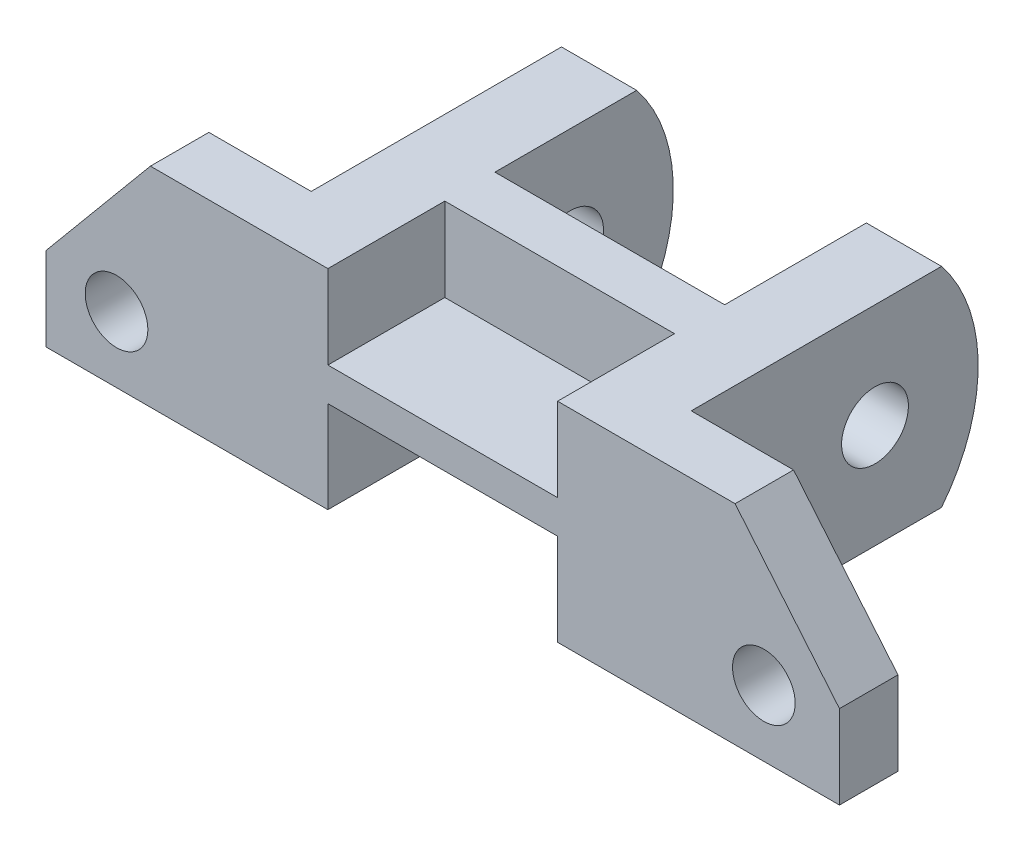
ISO-10303-21;
HEADER;
FILE_DESCRIPTION(('STEP AP214'),'2;1');
FILE_NAME('part.step','',(''),(''),'','','');
FILE_SCHEMA(('AUTOMOTIVE_DESIGN { 1 0 10303 214 1 1 1 1 }'));
ENDSEC;
DATA;
#1=APPLICATION_CONTEXT('core data for automotive mechanical design processes');
#2=APPLICATION_PROTOCOL_DEFINITION('international standard','automotive_design',2000,#1);
#3=PRODUCT_CONTEXT('',#1,'mechanical');
#4=PRODUCT('Part','Part','',(#3));
#5=PRODUCT_RELATED_PRODUCT_CATEGORY('part','',(#4));
#6=PRODUCT_DEFINITION_FORMATION('','',#4);
#7=PRODUCT_DEFINITION_CONTEXT('part definition',#1,'design');
#8=PRODUCT_DEFINITION('design','',#6,#7);
#9=PRODUCT_DEFINITION_SHAPE('','',#8);
#10=(LENGTH_UNIT() NAMED_UNIT(*) SI_UNIT(.MILLI.,.METRE.));
#11=(NAMED_UNIT(*) PLANE_ANGLE_UNIT() SI_UNIT($,.RADIAN.));
#12=(NAMED_UNIT(*) SI_UNIT($,.STERADIAN.) SOLID_ANGLE_UNIT());
#13=UNCERTAINTY_MEASURE_WITH_UNIT(LENGTH_MEASURE(1.E-05),#10,'distance_accuracy_value','');
#14=(GEOMETRIC_REPRESENTATION_CONTEXT(3) GLOBAL_UNCERTAINTY_ASSIGNED_CONTEXT((#13)) GLOBAL_UNIT_ASSIGNED_CONTEXT((#10,
#11,#12)) REPRESENTATION_CONTEXT('',''));
#15=CARTESIAN_POINT('',(0.,0.,0.));
#16=DIRECTION('',(0.,0.,1.));
#17=DIRECTION('',(1.,0.,0.));
#18=AXIS2_PLACEMENT_3D('',#15,#16,#17);
#19=CARTESIAN_POINT('',(0.,0.,14.));
#20=DIRECTION('',(0.,0.,1.));
#21=DIRECTION('',(1.,0.,0.));
#22=AXIS2_PLACEMENT_3D('',#19,#20,#21);
#23=PLANE('',#22);
#24=DIRECTION('',(0.,-1.,0.));
#25=VECTOR('',#24,1.);
#26=CARTESIAN_POINT('',(28.1119892819993,22.,14.));
#27=LINE('',#26,#25);
#28=CARTESIAN_POINT('',(28.1119892819993,22.,14.));
#29=VERTEX_POINT('',#28);
#30=CARTESIAN_POINT('',(28.1119892819993,0.,14.));
#31=VERTEX_POINT('',#30);
#32=EDGE_CURVE('E206',#29,#31,#27,.T.);
#33=ORIENTED_EDGE('',*,*,#32,.T.);
#34=DIRECTION('',(1.,0.,0.));
#35=VECTOR('',#34,1.);
#36=CARTESIAN_POINT('',(-94.3880107180007,0.,14.));
#37=LINE('',#36,#35);
#38=CARTESIAN_POINT('',(95.6119892819993,0.,14.));
#39=VERTEX_POINT('',#38);
#40=EDGE_CURVE('E326',#31,#39,#37,.T.);
#41=ORIENTED_EDGE('',*,*,#40,.T.);
#42=DIRECTION('',(0.,1.,0.));
#43=VECTOR('',#42,1.);
#44=CARTESIAN_POINT('',(95.6119892819993,0.,14.));
#45=LINE('',#44,#43);
#46=CARTESIAN_POINT('',(95.6119892819993,20.,14.));
#47=VERTEX_POINT('',#46);
#48=EDGE_CURVE('E332',#39,#47,#45,.T.);
#49=ORIENTED_EDGE('',*,*,#48,.T.);
#50=DIRECTION('',(-0.64018439966448,0.768221279597376,0.));
#51=VECTOR('',#50,1.);
#52=CARTESIAN_POINT('',(95.6119892819993,20.,14.));
#53=LINE('',#52,#51);
#54=CARTESIAN_POINT('',(70.6119892819993,50.,14.));
#55=VERTEX_POINT('',#54);
#56=EDGE_CURVE('E334',#47,#55,#53,.T.);
#57=ORIENTED_EDGE('',*,*,#56,.T.);
#58=DIRECTION('',(-1.,0.,0.));
#59=VECTOR('',#58,1.);
#60=CARTESIAN_POINT('',(70.6119892819993,50.,14.));
#61=LINE('',#60,#59);
#62=CARTESIAN_POINT('',(28.1119892819993,50.,14.));
#63=VERTEX_POINT('',#62);
#64=EDGE_CURVE('E337',#55,#63,#61,.T.);
#65=ORIENTED_EDGE('',*,*,#64,.T.);
#66=DIRECTION('',(0.,1.,0.));
#67=VECTOR('',#66,1.);
#68=CARTESIAN_POINT('',(28.1119892819993,30.,14.));
#69=LINE('',#68,#67);
#70=CARTESIAN_POINT('',(28.1119892819993,30.,14.));
#71=VERTEX_POINT('',#70);
#72=EDGE_CURVE('E244',#71,#63,#69,.T.);
#73=ORIENTED_EDGE('',*,*,#72,.F.);
#74=DIRECTION('',(1.,0.,0.));
#75=VECTOR('',#74,1.);
#76=CARTESIAN_POINT('',(0.,30.,14.));
#77=LINE('',#76,#75);
#78=CARTESIAN_POINT('',(-26.8880107180007,30.,14.));
#79=VERTEX_POINT('',#78);
#80=EDGE_CURVE('E233',#79,#71,#77,.T.);
#81=ORIENTED_EDGE('',*,*,#80,.F.);
#82=DIRECTION('',(0.,1.,0.));
#83=VECTOR('',#82,1.);
#84=CARTESIAN_POINT('',(-26.8880107180007,30.,14.));
#85=LINE('',#84,#83);
#86=CARTESIAN_POINT('',(-26.8880107180007,50.,14.));
#87=VERTEX_POINT('',#86);
#88=EDGE_CURVE('E249',#79,#87,#85,.T.);
#89=ORIENTED_EDGE('',*,*,#88,.T.);
#90=CARTESIAN_POINT('',(-69.3880107180007,50.,14.));
#91=VERTEX_POINT('',#90);
#92=EDGE_CURVE('E333',#87,#91,#61,.T.);
#93=ORIENTED_EDGE('',*,*,#92,.T.);
#94=DIRECTION('',(-0.64018439966448,-0.768221279597376,0.));
#95=VECTOR('',#94,1.);
#96=CARTESIAN_POINT('',(-69.3880107180007,50.,14.));
#97=LINE('',#96,#95);
#98=CARTESIAN_POINT('',(-94.3880107180007,20.,14.));
#99=VERTEX_POINT('',#98);
#100=EDGE_CURVE('E339',#91,#99,#97,.T.);
#101=ORIENTED_EDGE('',*,*,#100,.T.);
#102=DIRECTION('',(0.,-1.,0.));
#103=VECTOR('',#102,1.);
#104=CARTESIAN_POINT('',(-94.3880107180007,20.,14.));
#105=LINE('',#104,#103);
#106=CARTESIAN_POINT('',(-94.3880107180007,0.,14.));
#107=VERTEX_POINT('',#106);
#108=EDGE_CURVE('E323',#99,#107,#105,.T.);
#109=ORIENTED_EDGE('',*,*,#108,.T.);
#110=CARTESIAN_POINT('',(-26.8880107180007,0.,14.));
#111=VERTEX_POINT('',#110);
#112=EDGE_CURVE('E327',#107,#111,#37,.T.);
#113=ORIENTED_EDGE('',*,*,#112,.T.);
#114=DIRECTION('',(0.,-1.,0.));
#115=VECTOR('',#114,1.);
#116=CARTESIAN_POINT('',(-26.8880107180007,22.,14.));
#117=LINE('',#116,#115);
#118=CARTESIAN_POINT('',(-26.8880107180007,22.,14.));
#119=VERTEX_POINT('',#118);
#120=EDGE_CURVE('E54',#119,#111,#117,.T.);
#121=ORIENTED_EDGE('',*,*,#120,.F.);
#122=DIRECTION('',(1.,0.,0.));
#123=VECTOR('',#122,1.);
#124=CARTESIAN_POINT('',(0.,22.,14.));
#125=LINE('',#124,#123);
#126=EDGE_CURVE('E216',#119,#29,#125,.T.);
#127=ORIENTED_EDGE('',*,*,#126,.T.);
#128=EDGE_LOOP('',(#33,#41,#49,#57,#65,#73,#81,#89,#93,#101,#109,#113,#121,#127));
#129=FACE_BOUND('',#128,.T.);
#130=CARTESIAN_POINT('',(-77.5,15.7917491874742,14.));
#131=DIRECTION('',(0.,0.,1.));
#132=DIRECTION('',(1.,0.,0.));
#133=AXIS2_PLACEMENT_3D('',#130,#131,#132);
#134=CIRCLE('',#133,7.5);
#135=CARTESIAN_POINT('',(-70.,15.7917491874742,14.));
#136=VERTEX_POINT('',#135);
#137=EDGE_CURVE('E320',#136,#136,#134,.T.);
#138=ORIENTED_EDGE('',*,*,#137,.F.);
#139=EDGE_LOOP('',(#138));
#140=FACE_BOUND('',#139,.T.);
#141=CARTESIAN_POINT('',(77.5,15.7917491874742,14.));
#142=DIRECTION('',(0.,0.,1.));
#143=DIRECTION('',(1.,0.,0.));
#144=AXIS2_PLACEMENT_3D('',#141,#142,#143);
#145=CIRCLE('',#144,7.50000000000001);
#146=CARTESIAN_POINT('',(85.,15.7917491874742,14.));
#147=VERTEX_POINT('',#146);
#148=EDGE_CURVE('E313',#147,#147,#145,.T.);
#149=ORIENTED_EDGE('',*,*,#148,.F.);
#150=EDGE_LOOP('',(#149));
#151=FACE_BOUND('',#150,.T.);
#152=ADVANCED_FACE('F39',(#129,#140,#151),#23,.T.);
#153=CARTESIAN_POINT('',(70.6119892819993,50.,14.));
#154=DIRECTION('',(0.,-1.,0.));
#155=DIRECTION('',(1.,0.,0.));
#156=AXIS2_PLACEMENT_3D('',#153,#154,#155);
#157=PLANE('',#156);
#158=DIRECTION('',(0.,0.,1.));
#159=VECTOR('',#158,1.);
#160=CARTESIAN_POINT('',(28.1119892819993,50.,0.));
#161=LINE('',#160,#159);
#162=CARTESIAN_POINT('',(28.1119892819993,50.,-14.));
#163=VERTEX_POINT('',#162);
#164=EDGE_CURVE('E63',#163,#63,#161,.T.);
#165=ORIENTED_EDGE('',*,*,#164,.T.);
#166=ORIENTED_EDGE('',*,*,#64,.F.);
#167=DIRECTION('',(0.,0.,-1.));
#168=VECTOR('',#167,1.);
#169=CARTESIAN_POINT('',(70.6119892819993,50.,14.));
#170=LINE('',#169,#168);
#171=CARTESIAN_POINT('',(70.6119892819993,50.,0.));
#172=VERTEX_POINT('',#171);
#173=EDGE_CURVE('E362',#55,#172,#170,.T.);
#174=ORIENTED_EDGE('',*,*,#173,.T.);
#175=DIRECTION('',(-1.,0.,0.));
#176=VECTOR('',#175,1.);
#177=CARTESIAN_POINT('',(70.6119892819993,50.,0.));
#178=LINE('',#177,#176);
#179=CARTESIAN_POINT('',(46.1119892819993,50.,0.));
#180=VERTEX_POINT('',#179);
#181=EDGE_CURVE('E353',#172,#180,#178,.T.);
#182=ORIENTED_EDGE('',*,*,#181,.T.);
#183=DIRECTION('',(0.,0.,-1.));
#184=VECTOR('',#183,1.);
#185=CARTESIAN_POINT('',(46.1119892819993,50.,0.));
#186=LINE('',#185,#184);
#187=CARTESIAN_POINT('',(46.1119892819993,50.,-59.9340246594551));
#188=VERTEX_POINT('',#187);
#189=EDGE_CURVE('E301',#180,#188,#186,.T.);
#190=ORIENTED_EDGE('',*,*,#189,.T.);
#191=DIRECTION('',(1.,0.,0.));
#192=VECTOR('',#191,1.);
#193=CARTESIAN_POINT('',(-94.3880107180008,50.,-59.9340246594551));
#194=LINE('',#193,#192);
#195=CARTESIAN_POINT('',(28.1119892819993,50.,-59.9340246594551));
#196=VERTEX_POINT('',#195);
#197=EDGE_CURVE('E259',#196,#188,#194,.T.);
#198=ORIENTED_EDGE('',*,*,#197,.F.);
#199=DIRECTION('',(0.,0.,-1.));
#200=VECTOR('',#199,1.);
#201=CARTESIAN_POINT('',(28.1119892819993,50.,-84.));
#202=LINE('',#201,#200);
#203=CARTESIAN_POINT('',(28.1119892819993,50.,-26.));
#204=VERTEX_POINT('',#203);
#205=EDGE_CURVE('E289',#204,#196,#202,.T.);
#206=ORIENTED_EDGE('',*,*,#205,.F.);
#207=DIRECTION('',(1.,0.,0.));
#208=VECTOR('',#207,1.);
#209=CARTESIAN_POINT('',(-26.8880107180007,50.,-26.));
#210=LINE('',#209,#208);
#211=CARTESIAN_POINT('',(-26.8880107180007,50.,-26.));
#212=VERTEX_POINT('',#211);
#213=EDGE_CURVE('E284',#212,#204,#210,.T.);
#214=ORIENTED_EDGE('',*,*,#213,.F.);
#215=DIRECTION('',(0.,0.,1.));
#216=VECTOR('',#215,1.);
#217=CARTESIAN_POINT('',(-26.8880107180007,50.,-84.));
#218=LINE('',#217,#216);
#219=CARTESIAN_POINT('',(-26.8880107180007,50.,-59.934024659455));
#220=VERTEX_POINT('',#219);
#221=EDGE_CURVE('E274',#220,#212,#218,.T.);
#222=ORIENTED_EDGE('',*,*,#221,.F.);
#223=CARTESIAN_POINT('',(-44.8880107180007,50.,-59.9340246594551));
#224=VERTEX_POINT('',#223);
#225=EDGE_CURVE('E263',#224,#220,#194,.T.);
#226=ORIENTED_EDGE('',*,*,#225,.F.);
#227=DIRECTION('',(0.,0.,1.));
#228=VECTOR('',#227,1.);
#229=CARTESIAN_POINT('',(-44.8880107180007,50.,0.));
#230=LINE('',#229,#228);
#231=CARTESIAN_POINT('',(-44.8880107180007,50.,0.));
#232=VERTEX_POINT('',#231);
#233=EDGE_CURVE('E293',#224,#232,#230,.T.);
#234=ORIENTED_EDGE('',*,*,#233,.T.);
#235=CARTESIAN_POINT('',(-69.3880107180007,50.,0.));
#236=VERTEX_POINT('',#235);
#237=EDGE_CURVE('E355',#232,#236,#178,.T.);
#238=ORIENTED_EDGE('',*,*,#237,.T.);
#239=DIRECTION('',(0.,0.,-1.));
#240=VECTOR('',#239,1.);
#241=CARTESIAN_POINT('',(-69.3880107180007,50.,14.));
#242=LINE('',#241,#240);
#243=EDGE_CURVE('E356',#91,#236,#242,.T.);
#244=ORIENTED_EDGE('',*,*,#243,.F.);
#245=ORIENTED_EDGE('',*,*,#92,.F.);
#246=DIRECTION('',(0.,0.,1.));
#247=VECTOR('',#246,1.);
#248=CARTESIAN_POINT('',(-26.8880107180007,50.,0.));
#249=LINE('',#248,#247);
#250=CARTESIAN_POINT('',(-26.8880107180007,50.,-14.));
#251=VERTEX_POINT('',#250);
#252=EDGE_CURVE('E226',#251,#87,#249,.T.);
#253=ORIENTED_EDGE('',*,*,#252,.F.);
#254=DIRECTION('',(1.,0.,0.));
#255=VECTOR('',#254,1.);
#256=CARTESIAN_POINT('',(0.,50.,-14.));
#257=LINE('',#256,#255);
#258=EDGE_CURVE('E238',#251,#163,#257,.T.);
#259=ORIENTED_EDGE('',*,*,#258,.T.);
#260=EDGE_LOOP('',(#165,#166,#174,#182,#190,#198,#206,#214,#222,#226,#234,#238,#244,#245,#253,#259));
#261=FACE_BOUND('',#260,.T.);
#262=ADVANCED_FACE('F403',(#261),#157,.F.);
#263=CARTESIAN_POINT('',(-44.8880107180007,-123.842642090679,0.));
#264=DIRECTION('',(-1.,0.,0.));
#265=DIRECTION('',(0.,-1.,0.));
#266=AXIS2_PLACEMENT_3D('',#263,#264,#265);
#267=PLANE('',#266);
#268=CARTESIAN_POINT('',(-44.8880107180007,25.,-28.7090346674631));
#269=DIRECTION('',(-1.,0.,0.));
#270=DIRECTION('',(0.,-1.,0.));
#271=AXIS2_PLACEMENT_3D('',#268,#269,#270);
#272=CIRCLE('',#271,40.);
#273=CARTESIAN_POINT('',(-44.8880107180007,0.,-59.9340246594551));
#274=VERTEX_POINT('',#273);
#275=EDGE_CURVE('E270',#274,#224,#272,.F.);
#276=ORIENTED_EDGE('',*,*,#275,.F.);
#277=DIRECTION('',(0.,0.,-1.));
#278=VECTOR('',#277,1.);
#279=CARTESIAN_POINT('',(-44.8880107180007,0.,0.));
#280=LINE('',#279,#278);
#281=CARTESIAN_POINT('',(-44.8880107180007,0.,0.));
#282=VERTEX_POINT('',#281);
#283=EDGE_CURVE('E298',#282,#274,#280,.T.);
#284=ORIENTED_EDGE('',*,*,#283,.F.);
#285=DIRECTION('',(0.,1.,0.));
#286=VECTOR('',#285,1.);
#287=CARTESIAN_POINT('',(-44.8880107180007,-123.842642090679,0.));
#288=LINE('',#287,#286);
#289=EDGE_CURVE('E307',#282,#232,#288,.T.);
#290=ORIENTED_EDGE('',*,*,#289,.T.);
#291=ORIENTED_EDGE('',*,*,#233,.F.);
#292=EDGE_LOOP('',(#276,#284,#290,#291));
#293=FACE_BOUND('',#292,.T.);
#294=CARTESIAN_POINT('',(-44.8880107180007,25.,-44.));
#295=DIRECTION('',(-1.,0.,0.));
#296=DIRECTION('',(0.,-1.,0.));
#297=AXIS2_PLACEMENT_3D('',#294,#295,#296);
#298=CIRCLE('',#297,8.00000000000002);
#299=CARTESIAN_POINT('',(-44.8880107180007,17.,-44.));
#300=VERTEX_POINT('',#299);
#301=EDGE_CURVE('E275',#300,#300,#298,.T.);
#302=ORIENTED_EDGE('',*,*,#301,.F.);
#303=EDGE_LOOP('',(#302));
#304=FACE_BOUND('',#303,.T.);
#305=ADVANCED_FACE('F389',(#293,#304),#267,.T.);
#306=CARTESIAN_POINT('',(46.1119892819993,-123.842642090679,0.));
#307=DIRECTION('',(1.,0.,0.));
#308=DIRECTION('',(0.,1.,0.));
#309=AXIS2_PLACEMENT_3D('',#306,#307,#308);
#310=PLANE('',#309);
#311=CARTESIAN_POINT('',(46.1119892819993,25.,-28.7090346674631));
#312=DIRECTION('',(1.,0.,0.));
#313=DIRECTION('',(0.,1.,0.));
#314=AXIS2_PLACEMENT_3D('',#311,#312,#313);
#315=CIRCLE('',#314,40.);
#316=CARTESIAN_POINT('',(46.1119892819993,0.,-59.9340246594551));
#317=VERTEX_POINT('',#316);
#318=EDGE_CURVE('E247',#188,#317,#315,.F.);
#319=ORIENTED_EDGE('',*,*,#318,.F.);
#320=ORIENTED_EDGE('',*,*,#189,.F.);
#321=DIRECTION('',(0.,1.,0.));
#322=VECTOR('',#321,1.);
#323=CARTESIAN_POINT('',(46.1119892819993,-123.842642090679,0.));
#324=LINE('',#323,#322);
#325=CARTESIAN_POINT('',(46.1119892819993,0.,0.));
#326=VERTEX_POINT('',#325);
#327=EDGE_CURVE('E299',#326,#180,#324,.T.);
#328=ORIENTED_EDGE('',*,*,#327,.F.);
#329=DIRECTION('',(0.,0.,1.));
#330=VECTOR('',#329,1.);
#331=CARTESIAN_POINT('',(46.1119892819993,0.,0.));
#332=LINE('',#331,#330);
#333=EDGE_CURVE('E297',#317,#326,#332,.T.);
#334=ORIENTED_EDGE('',*,*,#333,.F.);
#335=EDGE_LOOP('',(#319,#320,#328,#334));
#336=FACE_BOUND('',#335,.T.);
#337=CARTESIAN_POINT('',(46.1119892819993,25.,-44.));
#338=DIRECTION('',(1.,0.,0.));
#339=DIRECTION('',(0.,1.,0.));
#340=AXIS2_PLACEMENT_3D('',#337,#338,#339);
#341=CIRCLE('',#340,8.00000000000002);
#342=CARTESIAN_POINT('',(46.1119892819993,33.,-44.));
#343=VERTEX_POINT('',#342);
#344=EDGE_CURVE('E251',#343,#343,#341,.T.);
#345=ORIENTED_EDGE('',*,*,#344,.F.);
#346=EDGE_LOOP('',(#345));
#347=FACE_BOUND('',#346,.T.);
#348=ADVANCED_FACE('F416',(#336,#347),#310,.T.);
#349=CARTESIAN_POINT('',(-26.8880107180007,-79.9312204335703,-84.));
#350=DIRECTION('',(-1.,0.,0.));
#351=DIRECTION('',(0.,-1.,0.));
#352=AXIS2_PLACEMENT_3D('',#349,#350,#351);
#353=PLANE('',#352);
#354=DIRECTION('',(0.,0.,-1.));
#355=VECTOR('',#354,1.);
#356=CARTESIAN_POINT('',(-26.8880107180007,0.,-84.));
#357=LINE('',#356,#355);
#358=CARTESIAN_POINT('',(-26.8880107180007,0.,-26.));
#359=VERTEX_POINT('',#358);
#360=CARTESIAN_POINT('',(-26.8880107180007,0.,-59.9340246594551));
#361=VERTEX_POINT('',#360);
#362=EDGE_CURVE('E279',#359,#361,#357,.T.);
#363=ORIENTED_EDGE('',*,*,#362,.T.);
#364=CARTESIAN_POINT('',(-26.8880107180007,25.,-28.7090346674631));
#365=DIRECTION('',(-1.,0.,0.));
#366=DIRECTION('',(0.,-1.,0.));
#367=AXIS2_PLACEMENT_3D('',#364,#365,#366);
#368=CIRCLE('',#367,40.);
#369=EDGE_CURVE('E258',#361,#220,#368,.F.);
#370=ORIENTED_EDGE('',*,*,#369,.T.);
#371=ORIENTED_EDGE('',*,*,#221,.T.);
#372=DIRECTION('',(0.,1.,0.));
#373=VECTOR('',#372,1.);
#374=CARTESIAN_POINT('',(-26.8880107180007,-79.9312204335703,-26.));
#375=LINE('',#374,#373);
#376=EDGE_CURVE('E288',#359,#212,#375,.T.);
#377=ORIENTED_EDGE('',*,*,#376,.F.);
#378=EDGE_LOOP('',(#363,#370,#371,#377));
#379=FACE_BOUND('',#378,.T.);
#380=CARTESIAN_POINT('',(-26.8880107180007,25.,-44.));
#381=DIRECTION('',(-1.,0.,0.));
#382=DIRECTION('',(0.,-1.,0.));
#383=AXIS2_PLACEMENT_3D('',#380,#381,#382);
#384=CIRCLE('',#383,8.00000000000002);
#385=CARTESIAN_POINT('',(-26.8880107180007,17.,-44.));
#386=VERTEX_POINT('',#385);
#387=EDGE_CURVE('E267',#386,#386,#384,.T.);
#388=ORIENTED_EDGE('',*,*,#387,.T.);
#389=EDGE_LOOP('',(#388));
#390=FACE_BOUND('',#389,.T.);
#391=ADVANCED_FACE('F397',(#379,#390),#353,.F.);
#392=CARTESIAN_POINT('',(28.1119892819993,-79.9312204335703,-84.));
#393=DIRECTION('',(1.,0.,0.));
#394=DIRECTION('',(0.,0.,-1.));
#395=AXIS2_PLACEMENT_3D('',#392,#393,#394);
#396=PLANE('',#395);
#397=ORIENTED_EDGE('',*,*,#205,.T.);
#398=CARTESIAN_POINT('',(28.1119892819993,25.,-28.7090346674631));
#399=DIRECTION('',(1.,0.,0.));
#400=DIRECTION('',(0.,0.,-1.));
#401=AXIS2_PLACEMENT_3D('',#398,#399,#400);
#402=CIRCLE('',#401,40.);
#403=CARTESIAN_POINT('',(28.1119892819993,0.,-59.9340246594551));
#404=VERTEX_POINT('',#403);
#405=EDGE_CURVE('E11',#196,#404,#402,.F.);
#406=ORIENTED_EDGE('',*,*,#405,.T.);
#407=DIRECTION('',(0.,0.,1.));
#408=VECTOR('',#407,1.);
#409=CARTESIAN_POINT('',(28.1119892819993,0.,-84.));
#410=LINE('',#409,#408);
#411=CARTESIAN_POINT('',(28.1119892819993,0.,-26.));
#412=VERTEX_POINT('',#411);
#413=EDGE_CURVE('E277',#404,#412,#410,.T.);
#414=ORIENTED_EDGE('',*,*,#413,.T.);
#415=DIRECTION('',(0.,1.,0.));
#416=VECTOR('',#415,1.);
#417=CARTESIAN_POINT('',(28.1119892819993,-79.9312204335703,-26.));
#418=LINE('',#417,#416);
#419=EDGE_CURVE('E276',#412,#204,#418,.T.);
#420=ORIENTED_EDGE('',*,*,#419,.T.);
#421=EDGE_LOOP('',(#397,#406,#414,#420));
#422=FACE_BOUND('',#421,.T.);
#423=CARTESIAN_POINT('',(28.1119892819993,25.,-44.));
#424=DIRECTION('',(1.,0.,0.));
#425=DIRECTION('',(0.,0.,-1.));
#426=AXIS2_PLACEMENT_3D('',#423,#424,#425);
#427=CIRCLE('',#426,8.00000000000002);
#428=CARTESIAN_POINT('',(28.1119892819993,25.,-52.));
#429=VERTEX_POINT('',#428);
#430=EDGE_CURVE('E43',#429,#429,#427,.T.);
#431=ORIENTED_EDGE('',*,*,#430,.T.);
#432=EDGE_LOOP('',(#431));
#433=FACE_BOUND('',#432,.T.);
#434=ADVANCED_FACE('F409',(#422,#433),#396,.F.);
#435=CARTESIAN_POINT('',(0.,0.,0.));
#436=DIRECTION('',(0.,0.,1.));
#437=DIRECTION('',(1.,0.,0.));
#438=AXIS2_PLACEMENT_3D('',#435,#436,#437);
#439=PLANE('',#438);
#440=CARTESIAN_POINT('',(-77.5,15.7917491874742,0.));
#441=DIRECTION('',(0.,0.,1.));
#442=DIRECTION('',(1.,0.,0.));
#443=AXIS2_PLACEMENT_3D('',#440,#441,#442);
#444=CIRCLE('',#443,7.5);
#445=CARTESIAN_POINT('',(-70.,15.7917491874742,0.));
#446=VERTEX_POINT('',#445);
#447=EDGE_CURVE('E314',#446,#446,#444,.T.);
#448=ORIENTED_EDGE('',*,*,#447,.T.);
#449=EDGE_LOOP('',(#448));
#450=FACE_BOUND('',#449,.T.);
#451=ORIENTED_EDGE('',*,*,#289,.F.);
#452=DIRECTION('',(1.,0.,0.));
#453=VECTOR('',#452,1.);
#454=CARTESIAN_POINT('',(-94.3880107180007,0.,0.));
#455=LINE('',#454,#453);
#456=CARTESIAN_POINT('',(-94.3880107180007,0.,0.));
#457=VERTEX_POINT('',#456);
#458=EDGE_CURVE('E343',#457,#282,#455,.T.);
#459=ORIENTED_EDGE('',*,*,#458,.F.);
#460=DIRECTION('',(0.,-1.,0.));
#461=VECTOR('',#460,1.);
#462=CARTESIAN_POINT('',(-94.3880107180007,20.,0.));
#463=LINE('',#462,#461);
#464=CARTESIAN_POINT('',(-94.3880107180007,20.,0.));
#465=VERTEX_POINT('',#464);
#466=EDGE_CURVE('E319',#465,#457,#463,.T.);
#467=ORIENTED_EDGE('',*,*,#466,.F.);
#468=DIRECTION('',(-0.64018439966448,-0.768221279597376,0.));
#469=VECTOR('',#468,1.);
#470=CARTESIAN_POINT('',(-69.3880107180007,50.,0.));
#471=LINE('',#470,#469);
#472=EDGE_CURVE('E330',#236,#465,#471,.T.);
#473=ORIENTED_EDGE('',*,*,#472,.F.);
#474=ORIENTED_EDGE('',*,*,#237,.F.);
#475=EDGE_LOOP('',(#451,#459,#467,#473,#474));
#476=FACE_BOUND('',#475,.T.);
#477=ADVANCED_FACE('F382',(#450,#476),#439,.F.);
#478=CARTESIAN_POINT('',(95.6119892819993,0.,0.));
#479=VERTEX_POINT('',#478);
#480=EDGE_CURVE('E341',#326,#479,#455,.T.);
#481=ORIENTED_EDGE('',*,*,#480,.F.);
#482=ORIENTED_EDGE('',*,*,#327,.T.);
#483=ORIENTED_EDGE('',*,*,#181,.F.);
#484=DIRECTION('',(-0.64018439966448,0.768221279597376,0.));
#485=VECTOR('',#484,1.);
#486=CARTESIAN_POINT('',(95.6119892819993,20.,0.));
#487=LINE('',#486,#485);
#488=CARTESIAN_POINT('',(95.6119892819993,20.,0.));
#489=VERTEX_POINT('',#488);
#490=EDGE_CURVE('E348',#489,#172,#487,.T.);
#491=ORIENTED_EDGE('',*,*,#490,.F.);
#492=DIRECTION('',(0.,1.,0.));
#493=VECTOR('',#492,1.);
#494=CARTESIAN_POINT('',(95.6119892819993,0.,0.));
#495=LINE('',#494,#493);
#496=EDGE_CURVE('E346',#479,#489,#495,.T.);
#497=ORIENTED_EDGE('',*,*,#496,.F.);
#498=EDGE_LOOP('',(#481,#482,#483,#491,#497));
#499=FACE_BOUND('',#498,.T.);
#500=CARTESIAN_POINT('',(77.5,15.7917491874742,0.));
#501=DIRECTION('',(0.,0.,1.));
#502=DIRECTION('',(1.,0.,0.));
#503=AXIS2_PLACEMENT_3D('',#500,#501,#502);
#504=CIRCLE('',#503,7.50000000000001);
#505=CARTESIAN_POINT('',(85.,15.7917491874742,0.));
#506=VERTEX_POINT('',#505);
#507=EDGE_CURVE('E304',#506,#506,#504,.T.);
#508=ORIENTED_EDGE('',*,*,#507,.T.);
#509=EDGE_LOOP('',(#508));
#510=FACE_BOUND('',#509,.T.);
#511=ADVANCED_FACE('F421',(#499,#510),#439,.F.);
#512=CARTESIAN_POINT('',(-94.3880107180007,20.,14.));
#513=DIRECTION('',(1.,0.,0.));
#514=DIRECTION('',(0.,1.,0.));
#515=AXIS2_PLACEMENT_3D('',#512,#513,#514);
#516=PLANE('',#515);
#517=ORIENTED_EDGE('',*,*,#466,.T.);
#518=DIRECTION('',(0.,0.,-1.));
#519=VECTOR('',#518,1.);
#520=CARTESIAN_POINT('',(-94.3880107180007,0.,14.));
#521=LINE('',#520,#519);
#522=EDGE_CURVE('E48',#107,#457,#521,.T.);
#523=ORIENTED_EDGE('',*,*,#522,.F.);
#524=ORIENTED_EDGE('',*,*,#108,.F.);
#525=DIRECTION('',(0.,0.,-1.));
#526=VECTOR('',#525,1.);
#527=CARTESIAN_POINT('',(-94.3880107180007,20.,14.));
#528=LINE('',#527,#526);
#529=EDGE_CURVE('E342',#99,#465,#528,.T.);
#530=ORIENTED_EDGE('',*,*,#529,.T.);
#531=EDGE_LOOP('',(#517,#523,#524,#530));
#532=FACE_BOUND('',#531,.T.);
#533=ADVANCED_FACE('F41',(#532),#516,.F.);
#534=CARTESIAN_POINT('',(-94.3880107180007,0.,14.));
#535=DIRECTION('',(0.,1.,0.));
#536=DIRECTION('',(0.,0.,1.));
#537=AXIS2_PLACEMENT_3D('',#534,#535,#536);
#538=PLANE('',#537);
#539=ORIENTED_EDGE('',*,*,#40,.F.);
#540=DIRECTION('',(0.,0.,1.));
#541=VECTOR('',#540,1.);
#542=CARTESIAN_POINT('',(28.1119892819993,0.,0.));
#543=LINE('',#542,#541);
#544=CARTESIAN_POINT('',(28.1119892819993,0.,-14.));
#545=VERTEX_POINT('',#544);
#546=EDGE_CURVE('E219',#545,#31,#543,.T.);
#547=ORIENTED_EDGE('',*,*,#546,.F.);
#548=DIRECTION('',(1.,0.,0.));
#549=VECTOR('',#548,1.);
#550=CARTESIAN_POINT('',(0.,0.,-14.));
#551=LINE('',#550,#549);
#552=CARTESIAN_POINT('',(-26.8880107180007,0.,-14.));
#553=VERTEX_POINT('',#552);
#554=EDGE_CURVE('E197',#553,#545,#551,.T.);
#555=ORIENTED_EDGE('',*,*,#554,.F.);
#556=DIRECTION('',(0.,0.,1.));
#557=VECTOR('',#556,1.);
#558=CARTESIAN_POINT('',(-26.8880107180007,0.,0.));
#559=LINE('',#558,#557);
#560=EDGE_CURVE('E209',#553,#111,#559,.T.);
#561=ORIENTED_EDGE('',*,*,#560,.T.);
#562=ORIENTED_EDGE('',*,*,#112,.F.);
#563=ORIENTED_EDGE('',*,*,#522,.T.);
#564=ORIENTED_EDGE('',*,*,#458,.T.);
#565=ORIENTED_EDGE('',*,*,#283,.T.);
#566=DIRECTION('',(1.,0.,0.));
#567=VECTOR('',#566,1.);
#568=CARTESIAN_POINT('',(-94.3880107180007,0.,-59.9340246594551));
#569=LINE('',#568,#567);
#570=EDGE_CURVE('E260',#274,#361,#569,.T.);
#571=ORIENTED_EDGE('',*,*,#570,.T.);
#572=ORIENTED_EDGE('',*,*,#362,.F.);
#573=DIRECTION('',(-1.,0.,0.));
#574=VECTOR('',#573,1.);
#575=CARTESIAN_POINT('',(-26.8880107180007,0.,-26.));
#576=LINE('',#575,#574);
#577=EDGE_CURVE('E285',#412,#359,#576,.T.);
#578=ORIENTED_EDGE('',*,*,#577,.F.);
#579=ORIENTED_EDGE('',*,*,#413,.F.);
#580=EDGE_CURVE('E257',#404,#317,#569,.T.);
#581=ORIENTED_EDGE('',*,*,#580,.T.);
#582=ORIENTED_EDGE('',*,*,#333,.T.);
#583=ORIENTED_EDGE('',*,*,#480,.T.);
#584=DIRECTION('',(0.,0.,-1.));
#585=VECTOR('',#584,1.);
#586=CARTESIAN_POINT('',(95.6119892819993,0.,14.));
#587=LINE('',#586,#585);
#588=EDGE_CURVE('E366',#39,#479,#587,.T.);
#589=ORIENTED_EDGE('',*,*,#588,.F.);
#590=EDGE_LOOP('',(#539,#547,#555,#561,#562,#563,#564,#565,#571,#572,#578,#579,#581,#582,#583,#589));
#591=FACE_BOUND('',#590,.T.);
#592=ADVANCED_FACE('F374',(#591),#538,.F.);
#593=CARTESIAN_POINT('',(95.6119892819993,0.,14.));
#594=DIRECTION('',(-1.,0.,0.));
#595=DIRECTION('',(0.,0.,1.));
#596=AXIS2_PLACEMENT_3D('',#593,#594,#595);
#597=PLANE('',#596);
#598=ORIENTED_EDGE('',*,*,#496,.T.);
#599=DIRECTION('',(0.,0.,-1.));
#600=VECTOR('',#599,1.);
#601=CARTESIAN_POINT('',(95.6119892819993,20.,14.));
#602=LINE('',#601,#600);
#603=EDGE_CURVE('E364',#47,#489,#602,.T.);
#604=ORIENTED_EDGE('',*,*,#603,.F.);
#605=ORIENTED_EDGE('',*,*,#48,.F.);
#606=ORIENTED_EDGE('',*,*,#588,.T.);
#607=EDGE_LOOP('',(#598,#604,#605,#606));
#608=FACE_BOUND('',#607,.T.);
#609=ADVANCED_FACE('F432',(#608),#597,.F.);
#610=CARTESIAN_POINT('',(95.6119892819993,20.,14.));
#611=DIRECTION('',(-0.768221279597376,-0.64018439966448,0.));
#612=DIRECTION('',(0.64018439966448,-0.768221279597376,0.));
#613=AXIS2_PLACEMENT_3D('',#610,#611,#612);
#614=PLANE('',#613);
#615=ORIENTED_EDGE('',*,*,#490,.T.);
#616=ORIENTED_EDGE('',*,*,#173,.F.);
#617=ORIENTED_EDGE('',*,*,#56,.F.);
#618=ORIENTED_EDGE('',*,*,#603,.T.);
#619=EDGE_LOOP('',(#615,#616,#617,#618));
#620=FACE_BOUND('',#619,.T.);
#621=ADVANCED_FACE('F431',(#620),#614,.F.);
#622=CARTESIAN_POINT('',(-69.3880107180007,50.,14.));
#623=DIRECTION('',(0.768221279597376,-0.64018439966448,0.));
#624=DIRECTION('',(0.64018439966448,0.768221279597376,0.));
#625=AXIS2_PLACEMENT_3D('',#622,#623,#624);
#626=PLANE('',#625);
#627=ORIENTED_EDGE('',*,*,#472,.T.);
#628=ORIENTED_EDGE('',*,*,#529,.F.);
#629=ORIENTED_EDGE('',*,*,#100,.F.);
#630=ORIENTED_EDGE('',*,*,#243,.T.);
#631=EDGE_LOOP('',(#627,#628,#629,#630));
#632=FACE_BOUND('',#631,.T.);
#633=ADVANCED_FACE('F444',(#632),#626,.F.);
#634=CARTESIAN_POINT('',(-77.5,15.7917491874742,14.));
#635=DIRECTION('',(0.,0.,-1.));
#636=DIRECTION('',(-1.,0.,0.));
#637=AXIS2_PLACEMENT_3D('',#634,#635,#636);
#638=CYLINDRICAL_SURFACE('',#637,7.5);
#639=ORIENTED_EDGE('',*,*,#137,.T.);
#640=EDGE_LOOP('',(#639));
#641=FACE_BOUND('',#640,.T.);
#642=ORIENTED_EDGE('',*,*,#447,.F.);
#643=EDGE_LOOP('',(#642));
#644=FACE_BOUND('',#643,.T.);
#645=ADVANCED_FACE('F473',(#641,#644),#638,.F.);
#646=CARTESIAN_POINT('',(77.5,15.7917491874742,14.));
#647=DIRECTION('',(0.,0.,-1.));
#648=DIRECTION('',(-1.,0.,0.));
#649=AXIS2_PLACEMENT_3D('',#646,#647,#648);
#650=CYLINDRICAL_SURFACE('',#649,7.50000000000001);
#651=ORIENTED_EDGE('',*,*,#148,.T.);
#652=EDGE_LOOP('',(#651));
#653=FACE_BOUND('',#652,.T.);
#654=ORIENTED_EDGE('',*,*,#507,.F.);
#655=EDGE_LOOP('',(#654));
#656=FACE_BOUND('',#655,.T.);
#657=ADVANCED_FACE('F508',(#653,#656),#650,.F.);
#658=CARTESIAN_POINT('',(-26.8880107180007,-79.9312204335703,-26.));
#659=DIRECTION('',(0.,0.,1.));
#660=DIRECTION('',(1.,0.,0.));
#661=AXIS2_PLACEMENT_3D('',#658,#659,#660);
#662=PLANE('',#661);
#663=ORIENTED_EDGE('',*,*,#577,.T.);
#664=ORIENTED_EDGE('',*,*,#376,.T.);
#665=ORIENTED_EDGE('',*,*,#213,.T.);
#666=ORIENTED_EDGE('',*,*,#419,.F.);
#667=EDGE_LOOP('',(#663,#664,#665,#666));
#668=FACE_BOUND('',#667,.T.);
#669=ADVANCED_FACE('F402',(#668),#662,.F.);
#670=CARTESIAN_POINT('',(-94.3880107180007,25.,-28.7090346674631));
#671=DIRECTION('',(1.,0.,0.));
#672=DIRECTION('',(0.,1.,0.));
#673=AXIS2_PLACEMENT_3D('',#670,#671,#672);
#674=CYLINDRICAL_SURFACE('',#673,40.);
#675=ORIENTED_EDGE('',*,*,#197,.T.);
#676=ORIENTED_EDGE('',*,*,#318,.T.);
#677=ORIENTED_EDGE('',*,*,#580,.F.);
#678=ORIENTED_EDGE('',*,*,#405,.F.);
#679=EDGE_LOOP('',(#675,#676,#677,#678));
#680=FACE_BOUND('',#679,.T.);
#681=ADVANCED_FACE('F446',(#680),#674,.T.);
#682=CARTESIAN_POINT('',(-94.3880107180007,25.,-44.));
#683=DIRECTION('',(1.,0.,0.));
#684=DIRECTION('',(0.,1.,0.));
#685=AXIS2_PLACEMENT_3D('',#682,#683,#684);
#686=CYLINDRICAL_SURFACE('',#685,8.00000000000002);
#687=ORIENTED_EDGE('',*,*,#344,.T.);
#688=EDGE_LOOP('',(#687));
#689=FACE_BOUND('',#688,.T.);
#690=ORIENTED_EDGE('',*,*,#430,.F.);
#691=EDGE_LOOP('',(#690));
#692=FACE_BOUND('',#691,.T.);
#693=ADVANCED_FACE('F448',(#689,#692),#686,.F.);
#694=ORIENTED_EDGE('',*,*,#275,.T.);
#695=ORIENTED_EDGE('',*,*,#225,.T.);
#696=ORIENTED_EDGE('',*,*,#369,.F.);
#697=ORIENTED_EDGE('',*,*,#570,.F.);
#698=EDGE_LOOP('',(#694,#695,#696,#697));
#699=FACE_BOUND('',#698,.T.);
#700=ADVANCED_FACE('F443',(#699),#674,.T.);
#701=ORIENTED_EDGE('',*,*,#301,.T.);
#702=EDGE_LOOP('',(#701));
#703=FACE_BOUND('',#702,.T.);
#704=ORIENTED_EDGE('',*,*,#387,.F.);
#705=EDGE_LOOP('',(#704));
#706=FACE_BOUND('',#705,.T.);
#707=ADVANCED_FACE('F450',(#703,#706),#686,.F.);
#708=CARTESIAN_POINT('',(28.1119892819993,30.,0.));
#709=DIRECTION('',(-1.,0.,0.));
#710=DIRECTION('',(0.,-1.,0.));
#711=AXIS2_PLACEMENT_3D('',#708,#709,#710);
#712=PLANE('',#711);
#713=ORIENTED_EDGE('',*,*,#164,.F.);
#714=DIRECTION('',(0.,1.,0.));
#715=VECTOR('',#714,1.);
#716=CARTESIAN_POINT('',(28.1119892819993,30.,-14.));
#717=LINE('',#716,#715);
#718=CARTESIAN_POINT('',(28.1119892819993,30.,-14.));
#719=VERTEX_POINT('',#718);
#720=EDGE_CURVE('E236',#719,#163,#717,.T.);
#721=ORIENTED_EDGE('',*,*,#720,.F.);
#722=DIRECTION('',(0.,0.,1.));
#723=VECTOR('',#722,1.);
#724=CARTESIAN_POINT('',(28.1119892819993,30.,0.));
#725=LINE('',#724,#723);
#726=EDGE_CURVE('E230',#719,#71,#725,.T.);
#727=ORIENTED_EDGE('',*,*,#726,.T.);
#728=ORIENTED_EDGE('',*,*,#72,.T.);
#729=EDGE_LOOP('',(#713,#721,#727,#728));
#730=FACE_BOUND('',#729,.T.);
#731=ADVANCED_FACE('F453',(#730),#712,.T.);
#732=CARTESIAN_POINT('',(-26.8880107180007,30.,0.));
#733=DIRECTION('',(-1.,0.,0.));
#734=DIRECTION('',(0.,-1.,0.));
#735=AXIS2_PLACEMENT_3D('',#732,#733,#734);
#736=PLANE('',#735);
#737=ORIENTED_EDGE('',*,*,#252,.T.);
#738=ORIENTED_EDGE('',*,*,#88,.F.);
#739=DIRECTION('',(0.,0.,1.));
#740=VECTOR('',#739,1.);
#741=CARTESIAN_POINT('',(-26.8880107180007,30.,0.));
#742=LINE('',#741,#740);
#743=CARTESIAN_POINT('',(-26.8880107180007,30.,-14.));
#744=VERTEX_POINT('',#743);
#745=EDGE_CURVE('E234',#744,#79,#742,.T.);
#746=ORIENTED_EDGE('',*,*,#745,.F.);
#747=DIRECTION('',(0.,1.,0.));
#748=VECTOR('',#747,1.);
#749=CARTESIAN_POINT('',(-26.8880107180007,30.,-14.));
#750=LINE('',#749,#748);
#751=EDGE_CURVE('E248',#744,#251,#750,.T.);
#752=ORIENTED_EDGE('',*,*,#751,.T.);
#753=EDGE_LOOP('',(#737,#738,#746,#752));
#754=FACE_BOUND('',#753,.T.);
#755=ADVANCED_FACE('F603',(#754),#736,.F.);
#756=CARTESIAN_POINT('',(0.,30.,-14.));
#757=DIRECTION('',(0.,0.,1.));
#758=DIRECTION('',(1.,0.,0.));
#759=AXIS2_PLACEMENT_3D('',#756,#757,#758);
#760=PLANE('',#759);
#761=ORIENTED_EDGE('',*,*,#258,.F.);
#762=ORIENTED_EDGE('',*,*,#751,.F.);
#763=DIRECTION('',(1.,0.,0.));
#764=VECTOR('',#763,1.);
#765=CARTESIAN_POINT('',(0.,30.,-14.));
#766=LINE('',#765,#764);
#767=EDGE_CURVE('E229',#744,#719,#766,.T.);
#768=ORIENTED_EDGE('',*,*,#767,.T.);
#769=ORIENTED_EDGE('',*,*,#720,.T.);
#770=EDGE_LOOP('',(#761,#762,#768,#769));
#771=FACE_BOUND('',#770,.T.);
#772=ADVANCED_FACE('F613',(#771),#760,.T.);
#773=CARTESIAN_POINT('',(0.,30.,0.));
#774=DIRECTION('',(0.,1.,0.));
#775=DIRECTION('',(-1.,0.,0.));
#776=AXIS2_PLACEMENT_3D('',#773,#774,#775);
#777=PLANE('',#776);
#778=ORIENTED_EDGE('',*,*,#726,.F.);
#779=ORIENTED_EDGE('',*,*,#767,.F.);
#780=ORIENTED_EDGE('',*,*,#745,.T.);
#781=ORIENTED_EDGE('',*,*,#80,.T.);
#782=EDGE_LOOP('',(#778,#779,#780,#781));
#783=FACE_BOUND('',#782,.T.);
#784=ADVANCED_FACE('F621',(#783),#777,.T.);
#785=CARTESIAN_POINT('',(28.1119892819993,22.,0.));
#786=DIRECTION('',(1.,0.,0.));
#787=DIRECTION('',(0.,1.,0.));
#788=AXIS2_PLACEMENT_3D('',#785,#786,#787);
#789=PLANE('',#788);
#790=ORIENTED_EDGE('',*,*,#546,.T.);
#791=ORIENTED_EDGE('',*,*,#32,.F.);
#792=DIRECTION('',(0.,0.,1.));
#793=VECTOR('',#792,1.);
#794=CARTESIAN_POINT('',(28.1119892819993,22.,0.));
#795=LINE('',#794,#793);
#796=CARTESIAN_POINT('',(28.1119892819993,22.,-14.));
#797=VERTEX_POINT('',#796);
#798=EDGE_CURVE('E201',#797,#29,#795,.T.);
#799=ORIENTED_EDGE('',*,*,#798,.F.);
#800=DIRECTION('',(0.,-1.,0.));
#801=VECTOR('',#800,1.);
#802=CARTESIAN_POINT('',(28.1119892819993,22.,-14.));
#803=LINE('',#802,#801);
#804=EDGE_CURVE('E192',#797,#545,#803,.T.);
#805=ORIENTED_EDGE('',*,*,#804,.T.);
#806=EDGE_LOOP('',(#790,#791,#799,#805));
#807=FACE_BOUND('',#806,.T.);
#808=ADVANCED_FACE('F204',(#807),#789,.F.);
#809=CARTESIAN_POINT('',(0.,22.,-14.));
#810=DIRECTION('',(0.,0.,-1.));
#811=DIRECTION('',(-1.,0.,0.));
#812=AXIS2_PLACEMENT_3D('',#809,#810,#811);
#813=PLANE('',#812);
#814=ORIENTED_EDGE('',*,*,#554,.T.);
#815=ORIENTED_EDGE('',*,*,#804,.F.);
#816=DIRECTION('',(1.,0.,0.));
#817=VECTOR('',#816,1.);
#818=CARTESIAN_POINT('',(0.,22.,-14.));
#819=LINE('',#818,#817);
#820=CARTESIAN_POINT('',(-26.8880107180007,22.,-14.));
#821=VERTEX_POINT('',#820);
#822=EDGE_CURVE('E193',#821,#797,#819,.T.);
#823=ORIENTED_EDGE('',*,*,#822,.F.);
#824=DIRECTION('',(0.,-1.,0.));
#825=VECTOR('',#824,1.);
#826=CARTESIAN_POINT('',(-26.8880107180007,22.,-14.));
#827=LINE('',#826,#825);
#828=EDGE_CURVE('E199',#821,#553,#827,.T.);
#829=ORIENTED_EDGE('',*,*,#828,.T.);
#830=EDGE_LOOP('',(#814,#815,#823,#829));
#831=FACE_BOUND('',#830,.T.);
#832=ADVANCED_FACE('F195',(#831),#813,.F.);
#833=CARTESIAN_POINT('',(-26.8880107180007,22.,0.));
#834=DIRECTION('',(1.,0.,0.));
#835=DIRECTION('',(0.,1.,0.));
#836=AXIS2_PLACEMENT_3D('',#833,#834,#835);
#837=PLANE('',#836);
#838=ORIENTED_EDGE('',*,*,#560,.F.);
#839=ORIENTED_EDGE('',*,*,#828,.F.);
#840=DIRECTION('',(0.,0.,1.));
#841=VECTOR('',#840,1.);
#842=CARTESIAN_POINT('',(-26.8880107180007,22.,0.));
#843=LINE('',#842,#841);
#844=EDGE_CURVE('E212',#821,#119,#843,.T.);
#845=ORIENTED_EDGE('',*,*,#844,.T.);
#846=ORIENTED_EDGE('',*,*,#120,.T.);
#847=EDGE_LOOP('',(#838,#839,#845,#846));
#848=FACE_BOUND('',#847,.T.);
#849=ADVANCED_FACE('F651',(#848),#837,.T.);
#850=CARTESIAN_POINT('',(0.,22.,0.));
#851=DIRECTION('',(0.,1.,0.));
#852=DIRECTION('',(-1.,0.,0.));
#853=AXIS2_PLACEMENT_3D('',#850,#851,#852);
#854=PLANE('',#853);
#855=ORIENTED_EDGE('',*,*,#798,.T.);
#856=ORIENTED_EDGE('',*,*,#126,.F.);
#857=ORIENTED_EDGE('',*,*,#844,.F.);
#858=ORIENTED_EDGE('',*,*,#822,.T.);
#859=EDGE_LOOP('',(#855,#856,#857,#858));
#860=FACE_BOUND('',#859,.T.);
#861=ADVANCED_FACE('F213',(#860),#854,.F.);
#862=CLOSED_SHELL('',(#152,#262,#305,#348,#391,#434,#477,#511,#533,#592,#609,#621,#633,#645,
#657,#669,#681,#693,#700,#707,#731,#755,#772,#784,#808,#832,#849,#861));
#863=MANIFOLD_SOLID_BREP('B2',#862);
#864=ADVANCED_BREP_SHAPE_REPRESENTATION('',(#18,#863),#14);
#865=SHAPE_DEFINITION_REPRESENTATION(#9,#864);
ENDSEC;
END-ISO-10303-21;
